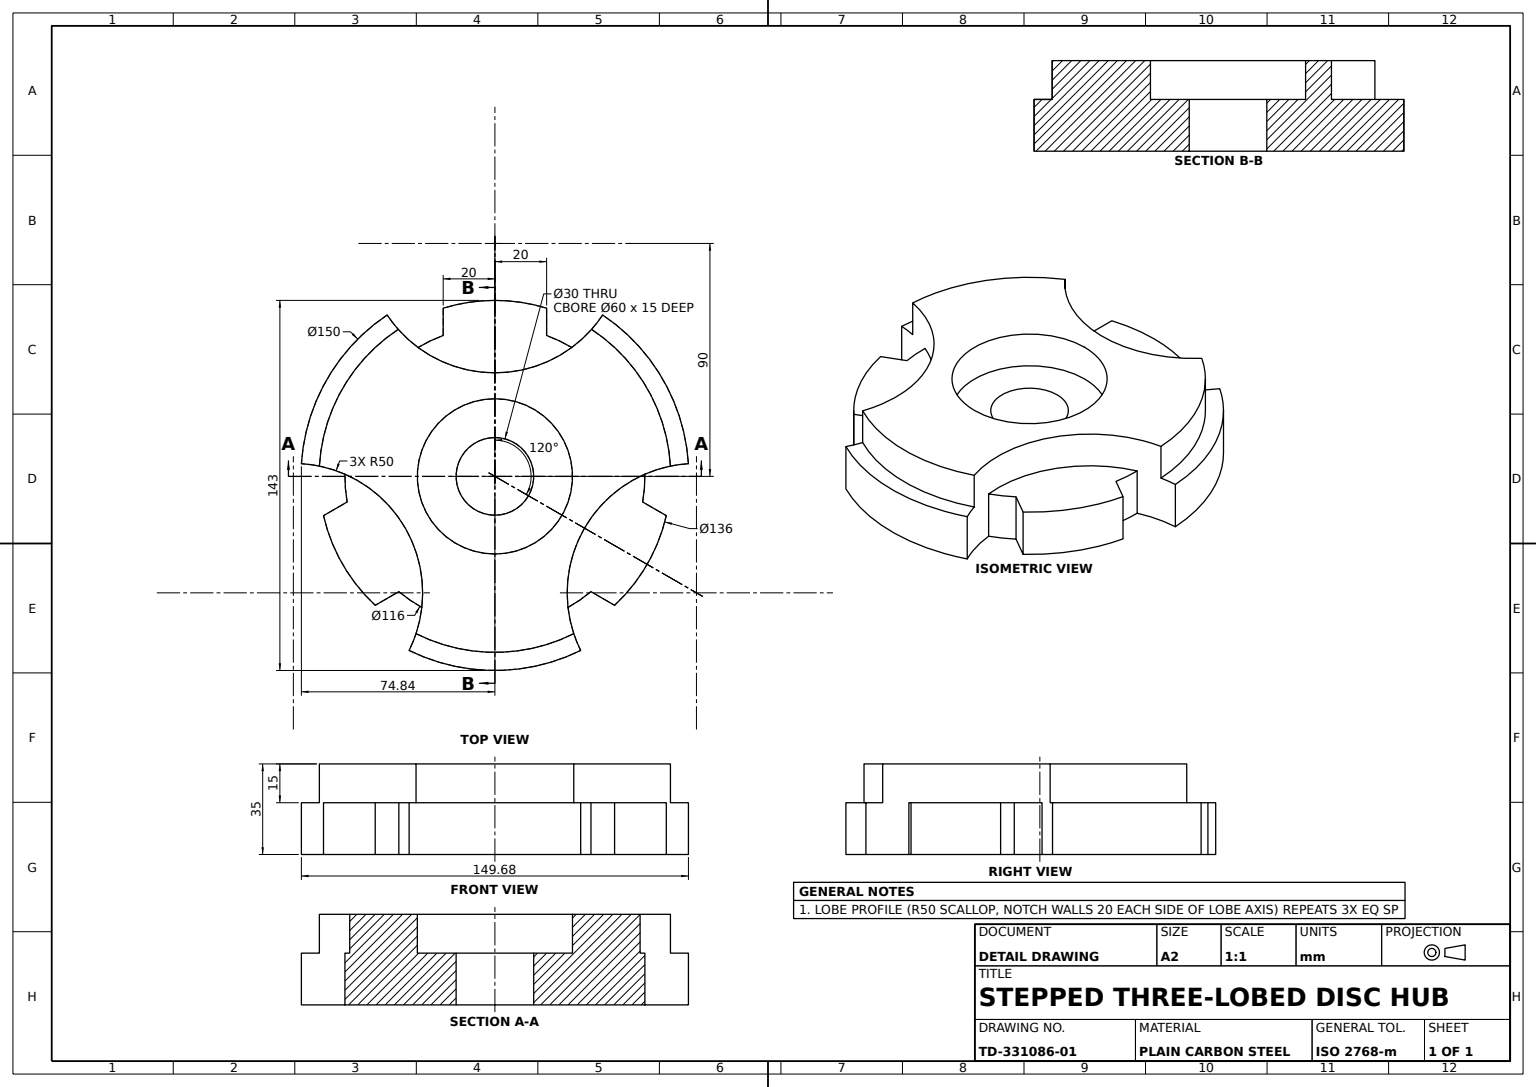
from build123d import *

# Parameters (mm, degrees)
BASE_LOBE_PLATE_20MM_DEPTH = 20
UPPER_LOBE_BOSS_15MM_DEPTH = 15
COUNTERBORE_SKETCH_60_R    = 30
COUNTERBORE_60X15_DEPTH    = 15
THROUGH_HOLE_SKETCH_30_R   = 15
THROUGH_HOLE_30_DEPTH      = 108.823718893


with BuildPart() as part:
    # Base Lobe Profile Sketch → Base Lobe Plate 20mm (new body)
    with BuildSketch(Plane(origin=(0, 0, 0), x_dir=(1, 0, 0), z_dir=(0, 1, 0))):
        with BuildLine():
            ThreePointArc((74.839524023, 4.903635799), (34.641016151, -20), (33.173088838, -67.264746911))
            ThreePointArc((33.173088838, -67.264746911), (0, -75), (-33.173088838, -67.264746911))
            ThreePointArc((-33.173088838, -67.264746911), (-34.641016151, -20), (-74.839524023, 4.903635799))
            ThreePointArc((-74.839524023, 4.903635799), (-64.951905284, 37.5), (-41.666435185, 62.361111111))
            ThreePointArc((-41.666435185, 62.361111111), (0, 40), (41.666435185, 62.361111111))
            ThreePointArc((41.666435185, 62.361111111), (64.951905284, 37.5), (74.839524023, 4.903635799))
        make_face()
        with BuildLine():
            ThreePointArc((-28.262332701, -50.648203821), (-34.641016151, -20), (-57.993797516, 0.848203821))
            ThreePointArc((-57.993797516, 0.848203821), (-57.821570771, -4.545982138), (-57.148700937, -9.900807102))
            Line((-57.148700937, -9.900807102), (-66.284989118, -15.175645543))
            ThreePointArc((-66.284989118, -15.175645543), (-58.889727457, -34), (-46.284989118, -49.816661694))
            Line((-46.284989118, -49.816661694), (-37.148700937, -44.541823253))
            ThreePointArc((-37.148700937, -44.541823253), (-32.847721402, -47.801958105), (-28.262332701, -50.648203821))
        make_face()
        with BuildLine():
            ThreePointArc((57.148700937, -9.900807102), (57.821570771, -4.545982138), (57.993797516, 0.848203821))
            ThreePointArc((57.993797516, 0.848203821), (34.641016151, -20), (28.262332701, -50.648203821))
            ThreePointArc((28.262332701, -50.648203821), (32.847721402, -47.801958105), (37.148700937, -44.541823253))
            Line((37.148700937, -44.541823253), (46.284989118, -49.816661694))
            ThreePointArc((46.284989118, -49.816661694), (58.889727457, -34), (66.284989118, -15.175645543))
            Line((66.284989118, -15.175645543), (57.148700937, -9.900807102))
        make_face()
        with BuildLine():
            ThreePointArc((29.731464814, 49.8), (24.973849369, 52.347940243), (20, 54.442630355))
            Line((20, 54.442630355), (20, 64.992307237))
            ThreePointArc((20, 64.992307237), (0, 68), (-20, 64.992307237))
            Line((-20, 64.992307237), (-20, 54.442630355))
            ThreePointArc((-20, 54.442630355), (-24.973849369, 52.347940243), (-29.731464814, 49.8))
            ThreePointArc((-29.731464814, 49.8), (0, 40), (29.731464814, 49.8))
        make_face()
    extrude(amount=BASE_LOBE_PLATE_20MM_DEPTH)

    # Upper Lobe Profile Sketch → Upper Lobe Boss 15mm (add)
    with BuildSketch(Plane(origin=(0, 20, 0), x_dir=(1, 0, 0), z_dir=(0, 1, 0))):
        with BuildLine():
            ThreePointArc((57.993797516, 0.848203821), (62.857299495, 2.670149694), (67.883557248, 3.977770152))
            ThreePointArc((67.883557248, 3.977770152), (58.889727457, 34), (37.386628626, 56.8))
            ThreePointArc((37.386628626, 56.8), (33.741067214, 53.100943329), (29.731464814, 49.8))
            ThreePointArc((29.731464814, 49.8), (0, 40), (-29.731464814, 49.8))
            ThreePointArc((-29.731464814, 49.8), (-33.741067214, 53.100943329), (-37.386628626, 56.8))
            ThreePointArc((-37.386628626, 56.8), (-58.889727457, 34), (-67.883557248, 3.977770152))
            ThreePointArc((-67.883557248, 3.977770152), (-62.857299495, 2.670149694), (-57.993797516, 0.848203821))
            ThreePointArc((-57.993797516, 0.848203821), (-34.641016151, -20), (-28.262332701, -50.648203821))
            ThreePointArc((-28.262332701, -50.648203821), (-29.11623228, -55.771093023), (-30.496928622, -60.777770152))
            ThreePointArc((-30.496928622, -60.777770152), (0, -68), (30.496928622, -60.777770152))
            ThreePointArc((30.496928622, -60.777770152), (29.11623228, -55.771093023), (28.262332701, -50.648203821))
            ThreePointArc((28.262332701, -50.648203821), (34.641016151, -20), (57.993797516, 0.848203821))
        make_face()
    extrude(amount=UPPER_LOBE_BOSS_15MM_DEPTH)

    # Counterbore Sketch Ø60 → Counterbore Ø60x15 (cut)
    with BuildSketch(Plane(origin=(0, 35, 0), x_dir=(1, 0, 0), z_dir=(0, 1, 0))):
        with Locations(Location((0, 0, 0), (0, 0, 270))):
            Circle(COUNTERBORE_SKETCH_60_R)
    extrude(amount=-COUNTERBORE_60X15_DEPTH, mode=Mode.SUBTRACT)

    # Through Hole Sketch Ø30 → Through Hole Ø30 (cut, through all)
    with BuildSketch(Plane(origin=(0, 20, 0), x_dir=(1, 0, 0), z_dir=(0, 1, 0))):
        with Locations(Location((0, 0, 0), (0, 0, 270))):
            Circle(THROUGH_HOLE_SKETCH_30_R)
    extrude(amount=-THROUGH_HOLE_30_DEPTH, mode=Mode.SUBTRACT)


solid = part.part
